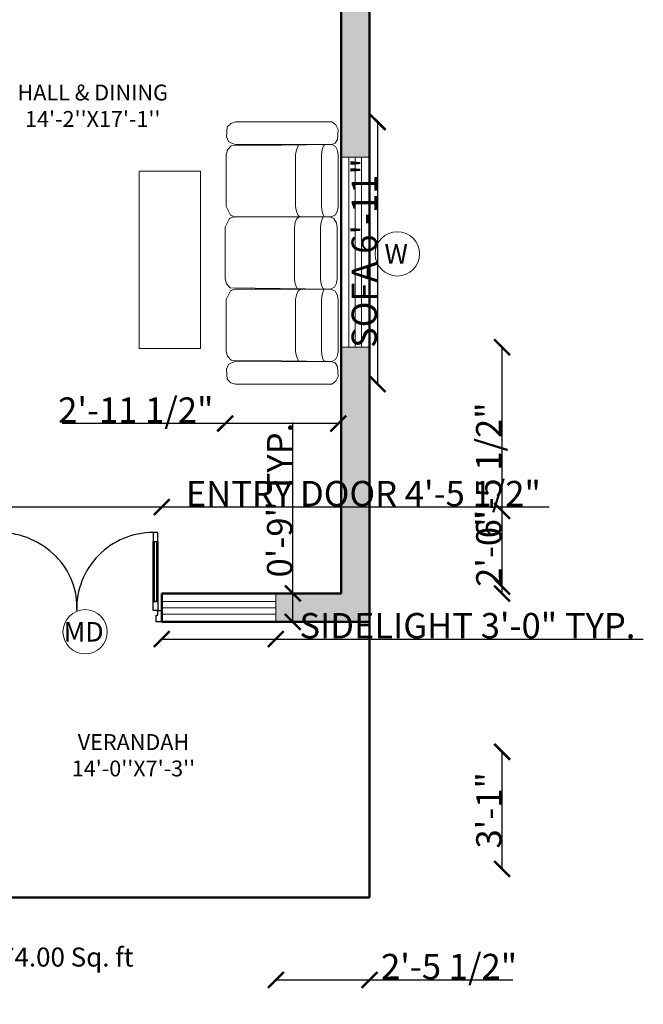
# Model space of a CAD drawing. Units: inches. Extents: x 1938 to 2373, y 1634 to 2225.
# Tile 3 of 5: x 2166 to 2363, y 1634 to 1945. Entities that reach past the tile are written whole.
import ezdxf

# ---------------------------------------------------------------- set-up
doc = ezdxf.new("R2010")
doc.units = ezdxf.units.IN
for name, color, linetype, lineweight in [('A-ANNO-DIMS', 2, 'Continuous', 18), ('A-ANNO-SYMB', 7, 'Continuous', 18), ('A-ANNO-TEXT', 7, 'Continuous', 18), ('A-AREA-IDEN', 7, 'Continuous', 18), ('A-FURN', 8, 'Continuous', 18), ('A-WALL-PATT', 82, 'Continuous', 13), ('MAIN DOOR', 150, 'Continuous', 25), ('WALL', 7, 'Continuous', 50), ('WINDOW', 150, 'Continuous', 18)]:
    doc.layers.add(name, color=color, linetype=linetype, lineweight=lineweight)
doc.layers.add('A-Glaz', color=92, linetype='Continuous')
doc.styles.get("Standard").update_dxf_attribs({"font": 'arial.ttf'})
doc.dimstyles.get("Standard").update_dxf_attribs({"dimtxt": 8, "dimasz": 5, "dimexe": 0.18, "dimexo": 0.0625, "dimgap": 0.09, "dimtad": 1, "dimdec": 1, "dimzin": 0, "dimdsep": 46, "dimlunit": 4, "dimtxsty": 'Standard', "dimblk": 'ARCHTICK', "dimcen": 0.09, "dimse1": 1, "dimse2": 1, "dimadec": 0, "dimazin": 0, "dimtfac": 1, "dimtdec": 1, "dimtofl": 0, "dimtmove": 0, "dimatfit": 3, "dimfxl": 1, "dimtolj": 1, "dimtzin": 0, "dimarcsym": 0})

# ---------------------------------------------------------------- blocks, each defined once
blk = doc.blocks.new('A$C13CE0A17')
at = {"layer": 'A-Glaz'}
for p, q in [((0.01, 0.61), (0.01, 0.08)), ((0.03, 0.08), (0.03, 0.61))]:
    blk.add_line(p, q, dxfattribs=at)
blk.add_lwpolyline([(1.4, 0.08), (1.4, 0.61), (1.42, 0.61), (1.42, 0.08)], close=True, dxfattribs=at)
at = {"layer": 'MAIN DOOR'}
for p, q in [((0, 0.61), (0, 0.69)), ((0, 0.69), (0.04, 0.69)), ((0, 0.61), (0, 0.08)), ((0.04, 0.61), (0, 0.61)), ((0.04, 0.61), (0, 0.61)), ((0.03, 0.61), (0.01, 0.61)), ((0.04, 0.69), (0.04, 0.61)), ((0.04, 0.08), (0.04, 0.61)), ((-0.035, 0), (-0.035, -0.1)), ((0, 0), (-0.035, 0)), ((0, 0.08), (0, 0)), ((0.04, 0.08), (0, 0.08)), ((0, 0.08), (0.04, 0.08)), ((0, 0), (0.04, 0)), ((0, -0.04), (0, 0)), ((0.01, 0.08), (0.03, 0.08)), ((0.04, 0), (0.04, 0.08)), ((0.015, -0.04), (0, -0.04)), ((0.015, -0.05), (0.015, -0.04)), ((0.015, -0.1), (0.015, -0.05)), ((-0.035, -0.1), (0.015, -0.1))]:
    blk.add_line(p, q, dxfattribs=at)
for points in [[(1.39, 0.69), (1.39, 0.61), (1.43, 0.61), (1.43, 0.69)], [(1.39, 0.08), (1.39, 0.61), (1.43, 0.61), (1.43, 0.08)], [(1.39, 0), (1.39, 0.08), (1.43, 0.08), (1.43, 0)], [(1.43, 0), (1.465, 0), (1.465, -0.1), (1.415, -0.1), (1.415, -0.05), (1.415, -0.04), (1.43, -0.04)]]:
    blk.add_lwpolyline(points, close=True, dxfattribs=at)
blk.add_arc((1.3872, 0.017), 0.673, 89.76573, 181.44381, dxfattribs=at)
blk.add_ellipse((0.0389, 0.0511), major_axis=(0.6669, -0.1217), ratio=0.940794, start_param=0.11153, end_param=1.73917, dxfattribs=at)
blk = doc.blocks.new('12PCOU17')
at = {"color": 0, "linetype": 'ByBlock'}
for points in [[(-34.71, 34.72), (-33.66, 34.31), (-3.27, 34.3), (-1.81, 34.76), (-1.05, 35.2), (-0.38, 36.65), (-0.61, 39.84), (-1.73, 40.94), (-3.27, 41.4), (-33.66, 41.4), (-34.95, 40.5), (-35.65, 39.02), (-35.49, 35.83), (-34.71, 34.72)], [(-1.89, 11.91), (-1.66, 11.91), (-0.35, 14.68), (-0.35, 31.05), (-0.74, 32.58), (-1.89, 33.83), (-33.63, 34.3), (-34.84, 33.63), (-35.43, 32.38), (-35.68, 31), (-35.68, 14.74), (-35.43, 13.36), (-34.66, 11.99), (-33.44, 11.43), (-3, 11.44), (-1.66, 11.91)], [(-31.25, 11.43), (-31.06, 11.84), (-30.6, 13.09), (-30.4, 14.62), (-30.4, 31.12), (-30.6, 32.65), (-31.06, 33.9), (-31.81, 34.3)], [(-23.84, 11.43), (-22.99, 11.9), (-22.46, 13.15), (-22.23, 14.67), (-22.23, 31.07), (-22.46, 32.59), (-22.99, 33.84), (-23.12, 34.3)], [(-1.54, -10.96), (-1.31, -10.96), (0, -8.19), (0, 8.19), (-0.39, 9.71), (-1.54, 10.96), (-33.28, 11.44), (-34.5, 10.77), (-35.08, 9.51), (-35.33, 8.14), (-35.33, -8.13), (-35.08, -9.51), (-34.31, -10.87), (-33.1, -11.44), (-2.65, -11.43), (-1.31, -10.96)], [(-30.9, -11.44), (-30.72, -11.02), (-30.25, -9.77), (-30.05, -8.25), (-30.05, 8.26), (-30.25, 9.78), (-30.72, 11.03), (-31.47, 11.44)], [(-23.49, -11.44), (-22.64, -10.96), (-22.11, -9.72), (-21.88, -8.19), (-21.88, 8.2), (-22.11, 9.73), (-22.64, 10.97), (-22.77, 11.44)], [(-1.89, -11.91), (-1.66, -11.91), (-0.35, -14.68), (-0.35, -31.05), (-0.74, -32.58), (-1.89, -33.83), (-33.63, -34.3), (-34.84, -33.63), (-35.43, -32.38), (-35.68, -31), (-35.68, -14.74), (-35.43, -13.36), (-34.66, -11.99), (-33.44, -11.43), (-3, -11.44), (-1.66, -11.91)], [(-31.25, -11.43), (-31.06, -11.84), (-30.6, -13.09), (-30.4, -14.62), (-30.4, -31.12), (-30.6, -32.65), (-31.06, -33.9), (-31.81, -34.3)], [(-23.84, -11.43), (-22.99, -11.9), (-22.46, -13.15), (-22.23, -14.67), (-22.23, -31.07), (-22.46, -32.59), (-22.99, -33.84), (-23.12, -34.3)], [(-34.71, -34.72), (-33.66, -34.31), (-3.27, -34.3), (-1.81, -34.76), (-1.05, -35.2), (-0.38, -36.65), (-0.61, -39.84), (-1.73, -40.94), (-3.27, -41.4), (-33.66, -41.4), (-34.95, -40.5), (-35.65, -39.02), (-35.49, -35.83), (-34.71, -34.72)]]:
    blk.add_lwpolyline(points, dxfattribs=at)
blk = doc.blocks.new('WIN-60IN')
for p, q in [((2.5, 0), (2.5, 60)), ((4.5, 0), (4.5, 60)), ((6.5, 0), (6.5, 60))]:
    blk.add_line(p, q)
blk.add_lwpolyline([(0, 0), (9, 0), (9, 60), (0, 60)], close=True)
blk = doc.blocks.new('WIN-36IN-SIDELIGHT')
for p, q in [((36, 6.5), (0, 6.5)), ((36, 4.5), (0, 4.5)), ((36, 2.5), (0, 2.5))]:
    blk.add_line(p, q)
blk.add_lwpolyline([(36, 0), (36, 9), (0, 9), (0, 0)], close=True)
blk = doc.blocks.new('TAG-WINDOW-W')
blk.add_circle((7, 7), 7)
blk.add_text('W', height=6.17).set_placement((2.93, 3.92))
blk = doc.blocks.new('_ArchTick')
at = {"color": 0, "linetype": 'ByBlock', "const_width": 0.15}
blk.add_lwpolyline([(-0.5, -0.5), (0.5, 0.5)], dxfattribs=at)
blk = doc.blocks.new('*D39')
at = {"layer": 'A-ANNO-DIMS', "color": 0, "lineweight": -2, "transparency": 16777216}
for p, q in [((2210.64, 1749.19), (2246.64, 1749.19)), ((2246.64, 1749.19), (2362.64, 1749.19))]:
    blk.add_line(p, q, dxfattribs=at)
at = {"layer": 'Defpoints', "color": 0, "transparency": 16777216}
for p in [(2210.64, 1754.59), (2246.64, 1754.59), (2246.64, 1749.19)]:
    blk.add_point(p, dxfattribs=at)
at = {"layer": 'A-ANNO-DIMS', "color": 0, "lineweight": -2, "transparency": 16777216, "xscale": 5, "yscale": 5, "zscale": 5, "rotation": 180}
blk.add_blockref('_ArchTick', (2210.64, 1749.19), dxfattribs=at)
at = {"layer": 'A-ANNO-DIMS', "color": 0, "lineweight": -2, "transparency": 16777216, "xscale": 5, "yscale": 5, "zscale": 5}
blk.add_blockref('_ArchTick', (2246.64, 1749.19), dxfattribs=at)
at = {"layer": 'A-ANNO-DIMS', "color": 0, "transparency": 16777216, "insert": (2307.14, 1753.41), "char_height": 8, "attachment_point": 5}
blk.add_mtext('\\A1;SIDELIGHT 3\'-0" TYP.', dxfattribs=at)
blk = doc.blocks.new('*D40')
at = {"layer": 'A-ANNO-DIMS', "color": 0, "lineweight": -2, "transparency": 16777216}
for p, q in [((2252.04, 1763.59), (2252.04, 1817.53)), ((2252.04, 1754.59), (2252.04, 1763.59))]:
    blk.add_line(p, q, dxfattribs=at)
at = {"layer": 'Defpoints', "color": 0, "transparency": 16777216}
for p in [(2246.64, 1763.59), (2252.04, 1763.59), (2246.64, 1754.59)]:
    blk.add_point(p, dxfattribs=at)
at = {"layer": 'A-ANNO-DIMS', "color": 0, "lineweight": -2, "transparency": 16777216, "xscale": 5, "yscale": 5, "zscale": 5}
for p, rotation in [((2252.04, 1763.59), 90), ((2252.04, 1754.59), 270)]:
    blk.add_blockref('_ArchTick', p, dxfattribs=dict(at, rotation=rotation))
at = {"layer": 'A-ANNO-DIMS', "color": 0, "transparency": 16777216, "insert": (2247.86, 1793.06), "char_height": 8, "attachment_point": 5, "rotation": 90}
blk.add_mtext('\\A1;0\'-9" TYP.', dxfattribs=at)
blk = doc.blocks.new('*D45')
at = {"layer": 'A-ANNO-DIMS', "color": 0, "lineweight": -2, "transparency": 16777216}
for p, q in [((2157.02, 1790.89), (2210.64, 1790.89)), ((2210.64, 1790.89), (2332.92, 1790.89))]:
    blk.add_line(p, q, dxfattribs=at)
at = {"layer": 'Defpoints', "color": 0, "transparency": 16777216}
for p in [(2210.64, 1790.89), (2157.02, 1782.85), (2210.64, 1782.85)]:
    blk.add_point(p, dxfattribs=at)
at = {"layer": 'A-ANNO-DIMS', "color": 0, "lineweight": -2, "transparency": 16777216, "xscale": 5, "yscale": 5, "zscale": 5, "rotation": 180}
blk.add_blockref('_ArchTick', (2157.02, 1790.89), dxfattribs=at)
at = {"layer": 'A-ANNO-DIMS', "color": 0, "lineweight": -2, "transparency": 16777216, "xscale": 5, "yscale": 5, "zscale": 5}
blk.add_blockref('_ArchTick', (2210.64, 1790.89), dxfattribs=at)
at = {"layer": 'A-ANNO-DIMS', "color": 0, "transparency": 16777216, "insert": (2274.28, 1795.12), "char_height": 8, "attachment_point": 5}
blk.add_mtext('\\A1;ENTRY DOOR 4\'-5 1/2"', dxfattribs=at)
blk = doc.blocks.new('*D49')
at = {"layer": 'A-ANNO-DIMS', "color": 0, "lineweight": -2, "transparency": 16777216}
blk.add_line((2278.78, 1912.49), (2278.78, 1829.69), dxfattribs=at)
at = {"layer": 'Defpoints', "color": 0, "transparency": 16777216}
for p in [(2266.36, 1912.49), (2266.36, 1829.69), (2278.78, 1829.69)]:
    blk.add_point(p, dxfattribs=at)
at = {"layer": 'A-ANNO-DIMS', "color": 0, "lineweight": -2, "transparency": 16777216, "xscale": 5, "yscale": 5, "zscale": 5}
for p, rotation in [((2278.78, 1912.49), 90), ((2278.78, 1829.69), 270)]:
    blk.add_blockref('_ArchTick', p, dxfattribs=dict(at, rotation=rotation))
at = {"layer": 'A-ANNO-DIMS', "color": 0, "transparency": 16777216, "insert": (2274.56, 1871.09), "char_height": 8, "attachment_point": 5, "rotation": 90}
blk.add_mtext('\\A1;SOFA 6\'-11"', dxfattribs=at)
blk = doc.blocks.new('*D50')
at = {"layer": 'A-ANNO-DIMS', "color": 0, "lineweight": -2, "transparency": 16777216}
for p, q in [((2230.68, 1817.27), (2179.24, 1817.27)), ((2266.36, 1817.27), (2230.68, 1817.27))]:
    blk.add_line(p, q, dxfattribs=at)
at = {"layer": 'Defpoints', "color": 0, "transparency": 16777216}
for p in [(2230.68, 1829.69), (2266.36, 1829.69), (2230.68, 1817.27)]:
    blk.add_point(p, dxfattribs=at)
at = {"layer": 'A-ANNO-DIMS', "color": 0, "lineweight": -2, "transparency": 16777216, "xscale": 5, "yscale": 5, "zscale": 5, "rotation": 180}
blk.add_blockref('_ArchTick', (2230.68, 1817.27), dxfattribs=at)
at = {"layer": 'A-ANNO-DIMS', "color": 0, "lineweight": -2, "transparency": 16777216, "xscale": 5, "yscale": 5, "zscale": 5}
blk.add_blockref('_ArchTick', (2266.36, 1817.27), dxfattribs=at)
at = {"layer": 'A-ANNO-DIMS', "color": 0, "transparency": 16777216, "insert": (2202.46, 1821.5), "char_height": 8, "attachment_point": 5}
blk.add_mtext('\\A1;2\'-11 1/2"', dxfattribs=at)
blk = doc.blocks.new('*D56')
at = {"layer": 'A-ANNO-DIMS', "color": 0, "lineweight": -2, "transparency": 16777216}
blk.add_line((2318.07, 1676.59), (2318.07, 1713.59), dxfattribs=at)
at = {"layer": 'Defpoints', "color": 0, "transparency": 16777216}
for p in [(2108.23, 1713.59), (2318.07, 1713.59), (2108.23, 1676.59)]:
    blk.add_point(p, dxfattribs=at)
at = {"layer": 'A-ANNO-DIMS', "color": 0, "lineweight": -2, "transparency": 16777216, "xscale": 5, "yscale": 5, "zscale": 5}
for p, rotation in [((2318.07, 1713.59), 90), ((2318.07, 1676.59), 270)]:
    blk.add_blockref('_ArchTick', p, dxfattribs=dict(at, rotation=rotation))
at = {"layer": 'A-ANNO-DIMS', "color": 0, "transparency": 16777216, "insert": (2313.89, 1695.09), "char_height": 8, "attachment_point": 5, "rotation": 90}
blk.add_mtext('\\A1;3\'-1"', dxfattribs=at)
blk = doc.blocks.new('*D63')
at = {"layer": 'A-ANNO-DIMS', "color": 0, "lineweight": -2, "transparency": 16777216}
blk.add_line((2318.07, 1763.59), (2318.07, 1841.32), dxfattribs=at)
at = {"layer": 'Defpoints', "color": 0, "transparency": 16777216}
for p in [(2267.23, 1841.32), (2318.07, 1841.32), (2267.23, 1763.59)]:
    blk.add_point(p, dxfattribs=at)
at = {"layer": 'A-ANNO-DIMS', "color": 0, "lineweight": -2, "transparency": 16777216, "xscale": 5, "yscale": 5, "zscale": 5}
for p, rotation in [((2318.07, 1841.32), 90), ((2318.07, 1763.59), 270)]:
    blk.add_blockref('_ArchTick', p, dxfattribs=dict(at, rotation=rotation))
at = {"layer": 'A-ANNO-DIMS', "color": 0, "transparency": 16777216, "insert": (2313.84, 1802.45), "char_height": 8, "attachment_point": 5, "rotation": 90}
blk.add_mtext('\\A1;6\'-5 1/2"', dxfattribs=at)
blk = doc.blocks.new('*D65')
at = {"layer": 'A-ANNO-DIMS', "color": 0, "lineweight": -2, "transparency": 16777216}
for p, q in [((2246.64, 1641.54), (2276.23, 1641.54)), ((2276.23, 1641.54), (2321.45, 1641.54))]:
    blk.add_line(p, q, dxfattribs=at)
at = {"layer": 'Defpoints', "color": 0, "transparency": 16777216}
for p in [(2246.64, 1754.59), (2276.23, 1754.59), (2276.23, 1641.54)]:
    blk.add_point(p, dxfattribs=at)
at = {"layer": 'A-ANNO-DIMS', "color": 0, "lineweight": -2, "transparency": 16777216, "xscale": 5, "yscale": 5, "zscale": 5, "rotation": 180}
blk.add_blockref('_ArchTick', (2246.64, 1641.54), dxfattribs=at)
at = {"layer": 'A-ANNO-DIMS', "color": 0, "lineweight": -2, "transparency": 16777216, "xscale": 5, "yscale": 5, "zscale": 5}
blk.add_blockref('_ArchTick', (2276.23, 1641.54), dxfattribs=at)
at = {"layer": 'A-ANNO-DIMS', "color": 0, "transparency": 16777216, "insert": (2301.34, 1645.76), "char_height": 8, "attachment_point": 5}
blk.add_mtext('\\A1;2\'-5 1/2"', dxfattribs=at)
blk = doc.blocks.new('*D70')
at = {"layer": 'A-ANNO-DIMS', "color": 0, "lineweight": -2, "transparency": 16777216}
blk.add_line((2318.07, 1765.79), (2318.07, 1789.65), dxfattribs=at)
at = {"layer": 'Defpoints', "color": 0, "transparency": 16777216}
for p in [(2085.39, 1789.65), (2318.07, 1789.65), (2085.39, 1765.79)]:
    blk.add_point(p, dxfattribs=at)
at = {"layer": 'A-ANNO-DIMS', "color": 0, "lineweight": -2, "transparency": 16777216, "xscale": 5, "yscale": 5, "zscale": 5}
for p, rotation in [((2318.07, 1789.65), 90), ((2318.07, 1765.79), 270)]:
    blk.add_blockref('_ArchTick', p, dxfattribs=dict(at, rotation=rotation))
at = {"layer": 'A-ANNO-DIMS', "color": 0, "transparency": 16777216, "insert": (2313.89, 1777.72), "char_height": 8, "attachment_point": 5, "rotation": 90}
blk.add_mtext('\\A1;2\'-0"', dxfattribs=at)

msp = doc.modelspace()

# ---------------------------------------------------------------- hatches: boundary and pattern name
at = {"layer": 'A-WALL-PATT', "transparency": 33554585}
h = msp.add_hatch(color=256, dxfattribs=at)
h.dxf.hatch_style = 1
h.paths.add_polyline_path([(2076.23, 2123.59), (2000.23, 2123.59), (2000.23, 2078.59), (2009.23, 2078.59), (2009.23, 2078.85), (2009.23, 2114.59), (2076.23, 2114.59)])
h.paths.add_polyline_path([(2219.23, 2123.59), (2136.23, 2123.59), (2136.23, 2114.59), (2203.23, 2114.59), (2203.23, 2085.96), (2207.23, 2085.96), (2207.23, 2114.59), (2219.23, 2114.59)])
h.paths.add_polyline_path([(2276.23, 2123.59), (2255.23, 2123.59), (2255.23, 2114.59), (2262.62, 2114.59), (2267.23, 2114.59), (2267.23, 2050.59), (2203.23, 2050.59), (2203.23, 1978.59), (2207.23, 1978.59), (2207.23, 1984.65), (2207.23, 2046.59), (2267.23, 2046.59), (2267.23, 2032.59), (2276.23, 2032.59)])
h.paths.add_polyline_path([(2009.23, 2018.59), (2000.23, 2018.59), (2000.23, 1948.59), (2009.23, 1948.59), (2009.23, 1948.85), (2009.23, 1978.59), (2126.4, 1978.59), (2126.4, 1978.59), (2133.23, 1978.59), (2166.7, 1978.59), (2166.7, 1982.59), (2009.23, 1982.59)])
h.paths.add_polyline_path([(2276.23, 1996.59), (2267.23, 1996.59), (2267.23, 1982.59), (2237.23, 1982.59), (2237.23, 1978.59), (2267.23, 1978.59), (2267.23, 1901.32), (2276.23, 1901.32)])
h.paths.add_polyline_path([(2133.23, 1944.79), (2129.23, 1944.79), (2129.23, 1858.59), (2009.23, 1858.59), (2009.23, 1888.59), (2000.23, 1888.59), (2000.23, 1839.09), (2009.23, 1839.09), (2009.23, 1854.59), (2091.31, 1854.59), (2091.31, 1854.61), (2097.36, 1854.59), (2133.23, 1854.59)])
h.paths.add_polyline_path([(2121.02, 1763.59), (2097.23, 1763.59), (2097.23, 1824.61), (2093.23, 1824.61), (2093.23, 1763.59), (2009.23, 1763.59), (2009.23, 1779.09), (2000.23, 1779.09), (2000.23, 1739.59), (2009.23, 1739.59), (2009.23, 1754.59), (2121.02, 1754.59)])
h.paths.add_polyline_path([(2108.23, 1676.59), (2009.23, 1676.59), (2009.23, 1691.59), (2000.23, 1691.59), (2000.23, 1667.59), (2108.23, 1667.59)])
h.paths.add_polyline_path([(2276.23, 1841.32), (2267.23, 1841.32), (2267.23, 1763.59), (2246.64, 1763.59), (2246.64, 1754.59), (2276.23, 1754.59)])

# ---------------------------------------------------------------- linework, layer by layer
at = {"layer": 'A-ANNO-SYMB'}
msp.add_circle((2186.47, 1751.47), 7, dxfattribs=at)
at = {"layer": 'A-FURN'}
msp.add_lwpolyline([(2203.52, 1896.92), (2222.86, 1896.92), (2222.86, 1840.96), (2203.52, 1840.96)], close=True, dxfattribs=at)
at = {"layer": 'WALL'}
for p, q in [((2276.23, 2123.59), (2276.23, 1667.59)), ((2267.23, 1763.59), (2267.23, 1978.59)), ((2210.64, 1754.59), (2210.64, 1763.59)), ((2210.64, 1763.59), (2267.23, 1763.59)), ((2210.64, 1754.59), (2276.23, 1754.59)), ((2000.23, 1667.59), (2276.23, 1667.59))]:
    msp.add_line(p, q, dxfattribs=at)

# ---------------------------------------------------------------- block references
at = {"layer": 'A-ANNO-SYMB'}
msp.add_blockref('TAG-WINDOW-W', (2278.02, 1863.82), dxfattribs=at)
at = {"layer": 'A-FURN', "rotation": 180}
msp.add_blockref('12PCOU17', (2230.68, 1871.09), dxfattribs=at)
at = {"layer": 'MAIN DOOR', "xscale": 35.74477478846772, "yscale": 35.74477478846772, "zscale": 35.74477478846772}
msp.add_blockref('A$C13CE0A17', (2158.27, 1758.16), dxfattribs=at)
at = {"layer": 'WINDOW'}
for name, p in [('WIN-60IN', (2267.23, 1841.32)), ('WIN-36IN-SIDELIGHT', (2210.64, 1754.59))]:
    msp.add_blockref(name, p, dxfattribs=at)

# ---------------------------------------------------------------- texts
at = {"layer": 'A-ANNO-SYMB'}
msp.add_text('MD', height=6.166, dxfattribs=at).set_placement((2179.68, 1748.39))
at = {"layer": 'A-ANNO-TEXT', "insert": (2095.13, 1651.75), "char_height": 6, "attachment_point": 1}
msp.add_mtext_dynamic_manual_height_columns('\\pxqc;Built Up Area : 874.00 Sq. ft', width=110.651, gutter_width=30.83, heights=[0], dxfattribs=at)
at = {"layer": 'A-AREA-IDEN', "char_height": 5, "attachment_point": 1}
for s, insert in [("\\pxqc;HALL & DINING \\P14'-2''X17'-1''", (2157.11, 1924.28)), ("\\pxqc;VERANDAH\\P14'-0''X7'-3''", (2169.96, 1719.15))]:
    msp.add_mtext_dynamic_manual_height_columns(s, width=63.5129, gutter_width=30.83, heights=[0], dxfattribs=dict(at, insert=insert))

# ---------------------------------------------------------------- dimensions: what is measured, and where the dimension line sits
at = {"layer": 'A-ANNO-DIMS'}
for base, p1, p2, angle, text, picture, middle in [((2278.78, 1829.69), (2266.36, 1912.49), (2266.36, 1829.69), 270, 'SOFA <>', '*D49', (2274.56, 1871.09)), ((2252.04, 1763.59), (2246.64, 1754.59), (2246.64, 1763.59), 90, '<> TYP.', '*D40', (2247.86, 1793.06))]:
    dim = msp.add_linear_dim(base=base, p1=p1, p2=p2, angle=angle, text=text, dimstyle='Standard', override={"dimdec": 1, "dimlfac": 1, "dimrnd": 0, "dimzin": 1, "dimdsep": 46, "dimlunit": 4, "dimfrac": 2}, dxfattribs=at)
    dim.commit()
    dim.dimension.update_dxf_attribs({"geometry": picture, "text_midpoint": middle})
for base, p1, p2, angle, picture, middle in [((2318.07, 1841.32), (2267.23, 1763.59), (2267.23, 1841.32), 90, '*D63', (2313.84, 1802.45)), ((2230.68, 1817.27), (2266.36, 1829.69), (2230.68, 1829.69), 180, '*D50', (2202.46, 1821.5)), ((2318.07, 1789.65), (2085.39, 1765.79), (2085.39, 1789.65), 90, '*D70', (2313.89, 1777.72)), ((2318.07, 1713.59), (2108.23, 1676.59), (2108.23, 1713.59), 90, '*D56', (2313.89, 1695.09))]:
    dim = msp.add_linear_dim(base=base, p1=p1, p2=p2, angle=angle, dimstyle='Standard', override={"dimdec": 1, "dimlfac": 1, "dimrnd": 0, "dimzin": 1, "dimdsep": 46, "dimlunit": 4, "dimfrac": 2}, dxfattribs=at)
    dim.commit()
    dim.dimension.update_dxf_attribs({"geometry": picture, "text_midpoint": middle})
for base, p1, p2, text, picture, middle in [((2210.64, 1790.89), (2157.02, 1782.85), (2210.64, 1782.85), 'ENTRY DOOR <>', '*D45', (2274.28, 1795.12)), ((2246.64, 1749.19), (2210.64, 1754.59), (2246.64, 1754.59), 'SIDELIGHT <> TYP.', '*D39', (2307.14, 1753.41))]:
    dim = msp.add_linear_dim(base=base, p1=p1, p2=p2, text=text, dimstyle='Standard', override={"dimdec": 1, "dimlfac": 1, "dimrnd": 0, "dimzin": 1, "dimdsep": 46, "dimlunit": 4, "dimfrac": 2}, dxfattribs=at)
    dim.commit()
    dim.dimension.update_dxf_attribs({"geometry": picture, "text_midpoint": middle})
dim = msp.add_linear_dim(base=(2276.23, 1641.54), p1=(2246.64, 1754.59), p2=(2276.23, 1754.59), dimstyle='Standard', override={"dimdec": 1, "dimlfac": 1, "dimrnd": 0, "dimzin": 1, "dimdsep": 46, "dimlunit": 4, "dimfrac": 2}, dxfattribs=at)
dim.commit()
dim.dimension.update_dxf_attribs({"geometry": '*D65', "text_midpoint": (2301.34, 1645.76)})

doc.saveas('drawing.dxf')
